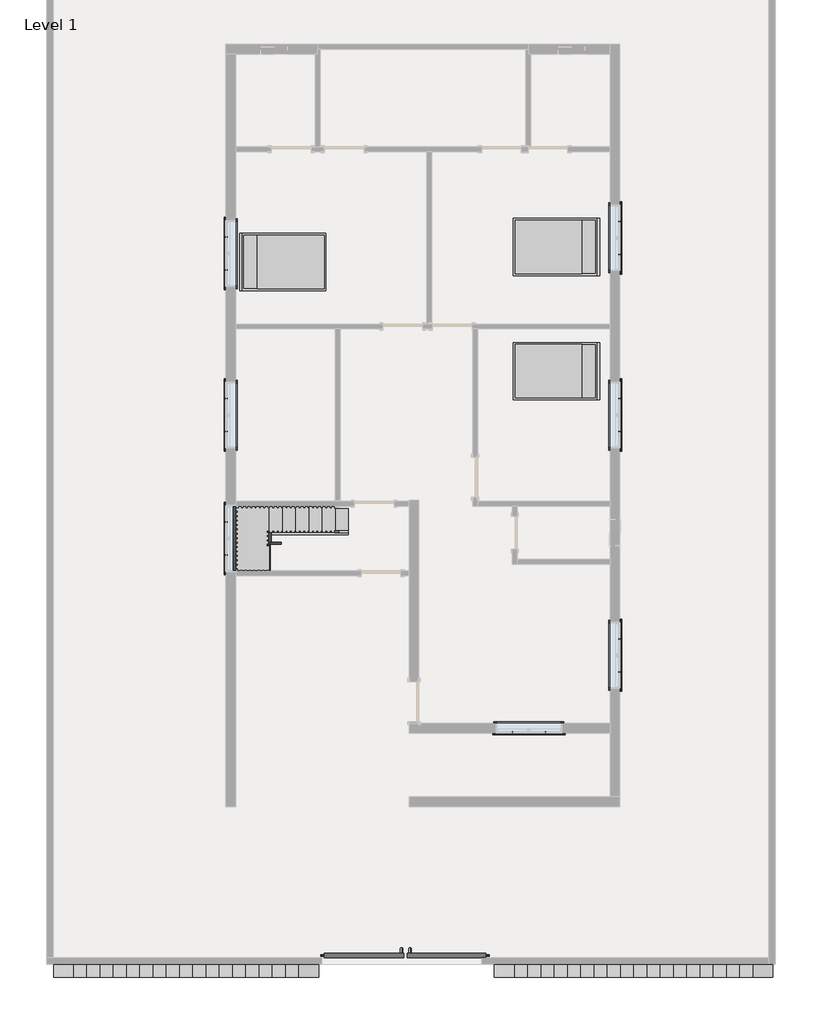
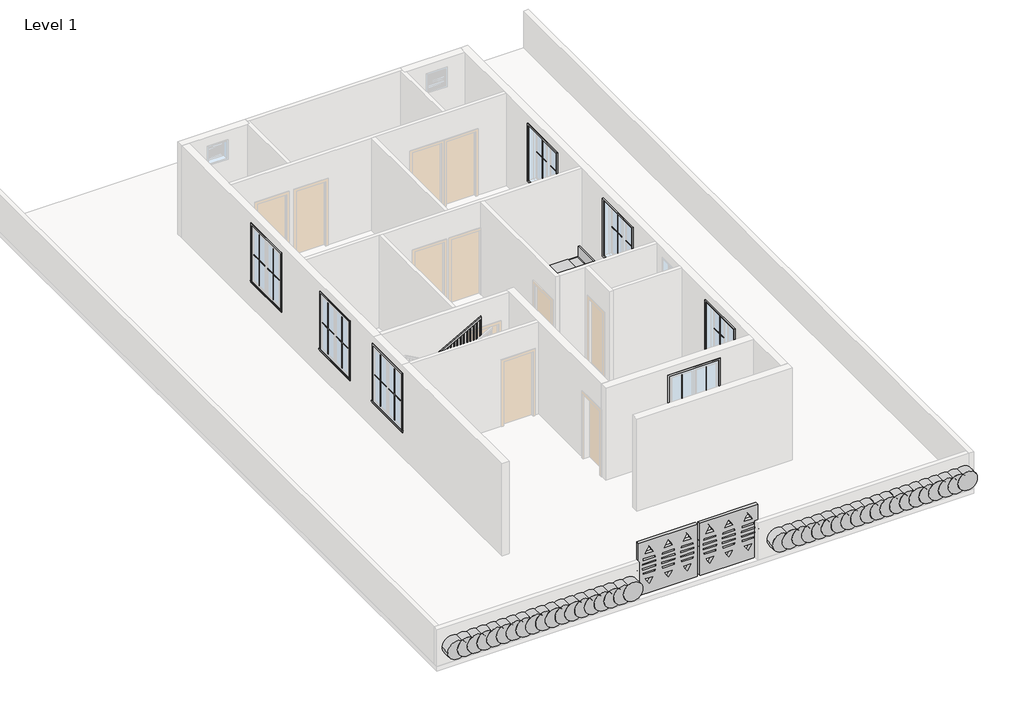
# One storey, part 3 of 3: 30 proxies, 6 members, 3 furniture elements, 1 railing, 1 stair flight.
"""IFC4 building model written with IfcOpenShell, lengths in millimetres."""

from ifc_helpers import new_model, si_unit, frame, origin, place, context, project, spatial, polyline, outline, extrude, faceted_brep, transform, mapped, element, save
from components import generic_models_477b0933, generic_models_1_generic_models_1_03ad02fd, muntin_pattern_2x2_muntin_pattern_2x2_f6a80940, muntin_pattern_2x2_muntin_pattern_2x2_09b00a1c, trim_window_exterior_flat_with_sill_698ed857, trim_window_interior_flat_picture_frame_92551a5e, bed_17739_bed_17739_15c61121, stair_flight_79800fe3

model = new_model("IFC4")

# Units and contexts
model_context = context("Model", 3, world=origin())
ifc_project = project(units=[si_unit("LENGTHUNIT", "METRE", prefix="MILLI")], contexts=[model_context])

# Site, building, storey
site = spatial("IfcSite", under=ifc_project)
building = spatial("IfcBuilding", under=site)
storey = spatial("IfcBuildingStorey", under=building, Name="Level 1", Elevation=0.0)

# Proxies
placement = place(None, origin())
generic_models_shape = generic_models_477b0933(model_context)
element("IfcBuildingElementProxy", 1, Name="Generic Models", at=placement, inside=storey, context=model_context, shape_type="MappedRepresentation", body=[
    mapped(generic_models_shape, transform((-1343.2120155, -12551.9052022, 0.0), x_axis=(-1.0, 0.0, 0.0), y_axis=(0.0, -1.0, 0.0), z_axis=(0.0, 0.0, 1.0))),
])
generic_models_1_generic_models_1_shape = generic_models_1_generic_models_1_03ad02fd(model_context)
element("IfcBuildingElementProxy", 2, Name="Generic Models 1 : Generic Models 1", ObjectType="Generic Models 1 : Generic Models 1", at=placement, inside=storey, context=model_context, shape_type="MappedRepresentation", body=[
    mapped(generic_models_1_generic_models_1_shape, transform((0.0, 0.0, 0.0), x_axis=(1.0, 0.0, 0.0), y_axis=(0.0, 1.0, 0.0), z_axis=(0.0, 0.0, 1.0))),
])
muntin_pattern_2x2_muntin_pattern_2x2_shape = muntin_pattern_2x2_muntin_pattern_2x2_f6a80940(model_context)
element("IfcBuildingElementProxy", 3, Name="Muntin Pattern_2x2 : Muntin Pattern_2x2", ObjectType="Muntin Pattern_2x2 : Muntin Pattern_2x2", at=placement, inside=storey, context=model_context, shape_type="MappedRepresentation", body=[
    mapped(muntin_pattern_2x2_muntin_pattern_2x2_shape, transform((-5778.6870155, 3260.8309309, 984.25), x_axis=(0.0, 1.0, 0.0), y_axis=(-1.0, 0.0, 0.0), z_axis=(0.0, 0.0, 1.0))),
])
element("IfcBuildingElementProxy", 4, Name="Muntin Pattern_2x2 : Muntin Pattern_2x2", ObjectType="Muntin Pattern_2x2 : Muntin Pattern_2x2", at=placement, inside=storey, context=model_context, shape_type="MappedRepresentation", body=[
    mapped(muntin_pattern_2x2_muntin_pattern_2x2_shape, transform((3270.0629845, 4381.6059309, 984.25), x_axis=(0.0, -1.0, 0.0), y_axis=(1.0, 0.0, 0.0), z_axis=(0.0, 0.0, 1.0))),
])
element("IfcBuildingElementProxy", 5, Name="Muntin Pattern_2x2 : Muntin Pattern_2x2", ObjectType="Muntin Pattern_2x2 : Muntin Pattern_2x2", at=placement, inside=storey, context=model_context, shape_type="MappedRepresentation", body=[
    mapped(muntin_pattern_2x2_muntin_pattern_2x2_shape, transform((3270.0629845, 304.9059309, 984.25), x_axis=(0.0, -1.0, 0.0), y_axis=(1.0, 0.0, 0.0), z_axis=(0.0, 0.0, 1.0))),
])
element("IfcBuildingElementProxy", 6, Name="Muntin Pattern_2x2 : Muntin Pattern_2x2", ObjectType="Muntin Pattern_2x2 : Muntin Pattern_2x2", at=placement, inside=storey, context=model_context, shape_type="MappedRepresentation", body=[
    mapped(muntin_pattern_2x2_muntin_pattern_2x2_shape, transform((3270.0629845, -5219.5940691, 984.25), x_axis=(0.0, -1.0, 0.0), y_axis=(1.0, 0.0, 0.0), z_axis=(0.0, 0.0, 1.0))),
])
element("IfcBuildingElementProxy", 7, Name="Muntin Pattern_2x2 : Muntin Pattern_2x2", ObjectType="Muntin Pattern_2x2 : Muntin Pattern_2x2", at=placement, inside=storey, context=model_context, shape_type="MappedRepresentation", body=[
    mapped(muntin_pattern_2x2_muntin_pattern_2x2_shape, transform((1563.5004845, -7380.1815691, 984.25), x_axis=(-1.0, 0.0, 0.0), y_axis=(0.0, -1.0, 0.0), z_axis=(0.0, 0.0, 1.0))),
])
element("IfcBuildingElementProxy", 8, Name="Muntin Pattern_2x2 : Muntin Pattern_2x2", ObjectType="Muntin Pattern_2x2 : Muntin Pattern_2x2", at=placement, inside=storey, context=model_context, shape_type="MappedRepresentation", body=[
    mapped(muntin_pattern_2x2_muntin_pattern_2x2_shape, transform((-5778.6870155, -3292.3690691, 984.25), x_axis=(0.0, 1.0, 0.0), y_axis=(-1.0, 0.0, 0.0), z_axis=(0.0, 0.0, 1.0))),
])
element("IfcBuildingElementProxy", 9, Name="Muntin Pattern_2x2 : Muntin Pattern_2x2", ObjectType="Muntin Pattern_2x2 : Muntin Pattern_2x2", at=placement, inside=storey, context=model_context, shape_type="MappedRepresentation", body=[
    mapped(muntin_pattern_2x2_muntin_pattern_2x2_shape, transform((-5778.6870155, -453.9190691, 984.25), x_axis=(0.0, 1.0, 0.0), y_axis=(-1.0, 0.0, 0.0), z_axis=(0.0, 0.0, 1.0))),
])
muntin_pattern_2x2_muntin_pattern_2x2_2_shape = muntin_pattern_2x2_muntin_pattern_2x2_09b00a1c(model_context)
element("IfcBuildingElementProxy", 10, Name="Muntin Pattern_2x2 : Muntin Pattern_2x2", ObjectType="Muntin Pattern_2x2 : Muntin Pattern_2x2", at=placement, inside=storey, context=model_context, shape_type="MappedRepresentation", body=[
    mapped(muntin_pattern_2x2_muntin_pattern_2x2_2_shape, transform((-5778.6870155, 4019.6559309, 984.25), x_axis=(0.0, -1.0, 0.0), y_axis=(1.0, 0.0, 0.0), z_axis=(0.0, 0.0, 1.0))),
])
element("IfcBuildingElementProxy", 11, Name="Muntin Pattern_2x2 : Muntin Pattern_2x2", ObjectType="Muntin Pattern_2x2 : Muntin Pattern_2x2", at=placement, inside=storey, context=model_context, shape_type="MappedRepresentation", body=[
    mapped(muntin_pattern_2x2_muntin_pattern_2x2_2_shape, transform((3270.0629845, 3622.7809309, 984.25), x_axis=(0.0, 1.0, 0.0), y_axis=(-1.0, 0.0, 0.0), z_axis=(0.0, 0.0, 1.0))),
])
element("IfcBuildingElementProxy", 12, Name="Muntin Pattern_2x2 : Muntin Pattern_2x2", ObjectType="Muntin Pattern_2x2 : Muntin Pattern_2x2", at=placement, inside=storey, context=model_context, shape_type="MappedRepresentation", body=[
    mapped(muntin_pattern_2x2_muntin_pattern_2x2_2_shape, transform((3270.0629845, -453.9190691, 984.25), x_axis=(0.0, 1.0, 0.0), y_axis=(-1.0, 0.0, 0.0), z_axis=(0.0, 0.0, 1.0))),
])
element("IfcBuildingElementProxy", 13, Name="Muntin Pattern_2x2 : Muntin Pattern_2x2", ObjectType="Muntin Pattern_2x2 : Muntin Pattern_2x2", at=placement, inside=storey, context=model_context, shape_type="MappedRepresentation", body=[
    mapped(muntin_pattern_2x2_muntin_pattern_2x2_2_shape, transform((3270.0629845, -5978.4190691, 984.25), x_axis=(0.0, 1.0, 0.0), y_axis=(-1.0, 0.0, 0.0), z_axis=(0.0, 0.0, 1.0))),
])
element("IfcBuildingElementProxy", 14, Name="Muntin Pattern_2x2 : Muntin Pattern_2x2", ObjectType="Muntin Pattern_2x2 : Muntin Pattern_2x2", at=placement, inside=storey, context=model_context, shape_type="MappedRepresentation", body=[
    mapped(muntin_pattern_2x2_muntin_pattern_2x2_2_shape, transform((804.6754845, -7380.1815691, 984.25), x_axis=(1.0, 0.0, 0.0), y_axis=(0.0, 1.0, 0.0), z_axis=(0.0, 0.0, 1.0))),
])
element("IfcBuildingElementProxy", 15, Name="Muntin Pattern_2x2 : Muntin Pattern_2x2", ObjectType="Muntin Pattern_2x2 : Muntin Pattern_2x2", at=placement, inside=storey, context=model_context, shape_type="MappedRepresentation", body=[
    mapped(muntin_pattern_2x2_muntin_pattern_2x2_2_shape, transform((-5778.6870155, -2533.5440691, 984.25), x_axis=(0.0, -1.0, 0.0), y_axis=(1.0, 0.0, 0.0), z_axis=(0.0, 0.0, 1.0))),
])
element("IfcBuildingElementProxy", 16, Name="Muntin Pattern_2x2 : Muntin Pattern_2x2", ObjectType="Muntin Pattern_2x2 : Muntin Pattern_2x2", at=placement, inside=storey, context=model_context, shape_type="MappedRepresentation", body=[
    mapped(muntin_pattern_2x2_muntin_pattern_2x2_2_shape, transform((-5778.6870155, 304.9059309, 984.25), x_axis=(0.0, -1.0, 0.0), y_axis=(1.0, 0.0, 0.0), z_axis=(0.0, 0.0, 1.0))),
])
trim_window_exterior_flat_with_sill_shape = trim_window_exterior_flat_with_sill_698ed857(model_context)
element("IfcBuildingElementProxy", 17, Name="Trim-Window-Exterior-Flat : with Sill", ObjectType="Trim-Window-Exterior-Flat : with Sill", at=placement, inside=storey, context=model_context, shape_type="MappedRepresentation", body=[
    mapped(trim_window_exterior_flat_with_sill_shape, transform((-5788.2120155, 3640.2434309, 2743.2), x_axis=(0.0, -1.0, 0.0), y_axis=(0.0, 0.0, 1.0), z_axis=(-1.0, 0.0, 0.0))),
])
element("IfcBuildingElementProxy", 18, Name="Trim-Window-Exterior-Flat : with Sill", ObjectType="Trim-Window-Exterior-Flat : with Sill", at=placement, inside=storey, context=model_context, shape_type="MappedRepresentation", body=[
    mapped(trim_window_exterior_flat_with_sill_shape, transform((3279.5879845, 4002.1934309, 2743.2), x_axis=(0.0, 1.0, 0.0), y_axis=(0.0, 0.0, 1.0), z_axis=(1.0, 0.0, 0.0))),
])
element("IfcBuildingElementProxy", 19, Name="Trim-Window-Exterior-Flat : with Sill", ObjectType="Trim-Window-Exterior-Flat : with Sill", at=placement, inside=storey, context=model_context, shape_type="MappedRepresentation", body=[
    mapped(trim_window_exterior_flat_with_sill_shape, transform((3279.5879845, -74.5065691, 2743.2), x_axis=(0.0, 1.0, 0.0), y_axis=(0.0, 0.0, 1.0), z_axis=(1.0, 0.0, 0.0))),
])
element("IfcBuildingElementProxy", 20, Name="Trim-Window-Exterior-Flat : with Sill", ObjectType="Trim-Window-Exterior-Flat : with Sill", at=placement, inside=storey, context=model_context, shape_type="MappedRepresentation", body=[
    mapped(trim_window_exterior_flat_with_sill_shape, transform((3279.5879845, -5599.0065691, 2743.2), x_axis=(0.0, 1.0, 0.0), y_axis=(0.0, 0.0, 1.0), z_axis=(1.0, 0.0, 0.0))),
])
element("IfcBuildingElementProxy", 21, Name="Trim-Window-Exterior-Flat : with Sill", ObjectType="Trim-Window-Exterior-Flat : with Sill", at=placement, inside=storey, context=model_context, shape_type="MappedRepresentation", body=[
    mapped(trim_window_exterior_flat_with_sill_shape, transform((1184.0879845, -7389.7065691, 2743.2), x_axis=(1.0, 0.0, 0.0), y_axis=(0.0, 0.0, 1.0), z_axis=(0.0, -1.0, 0.0))),
])
element("IfcBuildingElementProxy", 22, Name="Trim-Window-Exterior-Flat : with Sill", ObjectType="Trim-Window-Exterior-Flat : with Sill", at=placement, inside=storey, context=model_context, shape_type="MappedRepresentation", body=[
    mapped(trim_window_exterior_flat_with_sill_shape, transform((-5788.2120155, -2912.9565691, 2743.2), x_axis=(0.0, -1.0, 0.0), y_axis=(0.0, 0.0, 1.0), z_axis=(-1.0, 0.0, 0.0))),
])
element("IfcBuildingElementProxy", 23, Name="Trim-Window-Exterior-Flat : with Sill", ObjectType="Trim-Window-Exterior-Flat : with Sill", at=placement, inside=storey, context=model_context, shape_type="MappedRepresentation", body=[
    mapped(trim_window_exterior_flat_with_sill_shape, transform((-5788.2120155, -74.5065691, 2743.2), x_axis=(0.0, -1.0, 0.0), y_axis=(0.0, 0.0, 1.0), z_axis=(-1.0, 0.0, 0.0))),
])
trim_window_interior_flat_picture_frame_shape = trim_window_interior_flat_picture_frame_92551a5e(model_context)
element("IfcBuildingElementProxy", 24, Name="Trim-Window-Interior-Flat : Picture Frame", ObjectType="Trim-Window-Interior-Flat : Picture Frame", at=placement, inside=storey, context=model_context, shape_type="MappedRepresentation", body=[
    mapped(trim_window_interior_flat_picture_frame_shape, transform((-5559.6120155, 3640.2434309, 2743.2), x_axis=(0.0, 1.0, 0.0), y_axis=(0.0, 0.0, 1.0), z_axis=(1.0, 0.0, 0.0))),
])
element("IfcBuildingElementProxy", 25, Name="Trim-Window-Interior-Flat : Picture Frame", ObjectType="Trim-Window-Interior-Flat : Picture Frame", at=placement, inside=storey, context=model_context, shape_type="MappedRepresentation", body=[
    mapped(trim_window_interior_flat_picture_frame_shape, transform((3050.9879845, 4002.1934309, 2743.2), x_axis=(0.0, -1.0, 0.0), y_axis=(0.0, 0.0, 1.0), z_axis=(-1.0, 0.0, 0.0))),
])
element("IfcBuildingElementProxy", 26, Name="Trim-Window-Interior-Flat : Picture Frame", ObjectType="Trim-Window-Interior-Flat : Picture Frame", at=placement, inside=storey, context=model_context, shape_type="MappedRepresentation", body=[
    mapped(trim_window_interior_flat_picture_frame_shape, transform((3050.9879845, -74.5065691, 2743.2), x_axis=(0.0, -1.0, 0.0), y_axis=(0.0, 0.0, 1.0), z_axis=(-1.0, 0.0, 0.0))),
])
element("IfcBuildingElementProxy", 27, Name="Trim-Window-Interior-Flat : Picture Frame", ObjectType="Trim-Window-Interior-Flat : Picture Frame", at=placement, inside=storey, context=model_context, shape_type="MappedRepresentation", body=[
    mapped(trim_window_interior_flat_picture_frame_shape, transform((3050.9879845, -5599.0065691, 2743.2), x_axis=(0.0, -1.0, 0.0), y_axis=(0.0, 0.0, 1.0), z_axis=(-1.0, 0.0, 0.0))),
])
element("IfcBuildingElementProxy", 28, Name="Trim-Window-Interior-Flat : Picture Frame", ObjectType="Trim-Window-Interior-Flat : Picture Frame", at=placement, inside=storey, context=model_context, shape_type="MappedRepresentation", body=[
    mapped(trim_window_interior_flat_picture_frame_shape, transform((1184.0879845, -7161.1065691, 2743.2), x_axis=(-1.0, 0.0, 0.0), y_axis=(0.0, 0.0, 1.0), z_axis=(0.0, 1.0, 0.0))),
])
element("IfcBuildingElementProxy", 29, Name="Trim-Window-Interior-Flat : Picture Frame", ObjectType="Trim-Window-Interior-Flat : Picture Frame", at=placement, inside=storey, context=model_context, shape_type="MappedRepresentation", body=[
    mapped(trim_window_interior_flat_picture_frame_shape, transform((-5559.6120155, -2912.9565691, 2743.2), x_axis=(0.0, 1.0, 0.0), y_axis=(0.0, 0.0, 1.0), z_axis=(1.0, 0.0, 0.0))),
])
element("IfcBuildingElementProxy", 30, Name="Trim-Window-Interior-Flat : Picture Frame", ObjectType="Trim-Window-Interior-Flat : Picture Frame", at=placement, inside=storey, context=model_context, shape_type="MappedRepresentation", body=[
    mapped(trim_window_interior_flat_picture_frame_shape, transform((-5559.6120155, -74.5065691, 2743.2), x_axis=(0.0, 1.0, 0.0), y_axis=(0.0, 0.0, 1.0), z_axis=(1.0, 0.0, 0.0))),
])

# Furniture
bed_17739_bed_17739_shape = bed_17739_bed_17739_15c61121(model_context)
element("IfcFurniture", 31, ObjectType="Bed_17739 : Bed_17739", at=placement, inside=storey, context=model_context, shape_type="MappedRepresentation", body=[
    mapped(bed_17739_bed_17739_shape, transform((-4454.7120155, 3449.7434309, 0.0), x_axis=(0.0, 1.0, 0.0), y_axis=(-1.0, 0.0, 0.0), z_axis=(0.0, 0.0, 1.0))),
])
element("IfcFurniture", 32, ObjectType="Bed_17739 : Bed_17739", at=placement, inside=storey, context=model_context, shape_type="MappedRepresentation", body=[
    mapped(bed_17739_bed_17739_shape, transform((1793.6879845, 3792.6434309, 0.0), x_axis=(0.0, -1.0, 0.0), y_axis=(1.0, 0.0, 0.0), z_axis=(0.0, 0.0, 1.0))),
])
element("IfcFurniture", 33, ObjectType="Bed_17739 : Bed_17739", at=placement, inside=storey, context=model_context, shape_type="MappedRepresentation", body=[
    mapped(bed_17739_bed_17739_shape, transform((1793.6879845, 935.1434309, 0.0), x_axis=(0.0, -1.0, 0.0), y_axis=(1.0, 0.0, 0.0), z_axis=(0.0, 0.0, 1.0))),
])

# Members
element("IfcMember", 34, ObjectType="Stringer - 2\" Width", at=placement, inside=storey, context=model_context, shape_type="SweptSolid", body=[
    extrude(outline(polyline([(0.0, -2968.8120155), (207.5983948, -2968.8120155), (1195.3761726, -4746.8120155), (846.6974984, -4746.8120155), (0.0, -3222.7565183), (0.0, -2968.8120155)])), frame((0.0, -2830.4065691, 0.0), z_axis=(0.0, 1.0, 0.0), x_axis=(0.0, 0.0, 1.0)), (0.0, 0.0, 1.0), 50.8),
])
element("IfcMember", 35, ObjectType="Stringer - 2\" Width", at=placement, inside=storey, context=model_context, shape_type="SweptSolid", body=[
    extrude(outline(polyline([(-4797.6120155, -2779.6065691), (-4746.8120155, -2779.6065691), (-4746.8120155, -2995.5065691), (-4797.6120155, -2995.5065691), (-4797.6120155, -2779.6065691)])), frame((0.0, 0.0, 956.7333333), z_axis=(0.0, 0.0, 1.0), x_axis=(1.0, 0.0, 0.0)), (0.0, 0.0, 1.0), 304.8),
])
element("IfcMember", 36, ObjectType="Stringer - 2\" Width", at=placement, inside=storey, context=model_context, shape_type="SweptSolid", body=[
    extrude(outline(polyline([(1392.9317281, -4797.6120155), (1044.253054, -4797.6120155), (2060.253054, -2968.8120155), (2408.9317281, -2968.8120155), (1392.9317281, -4797.6120155)])), frame((0.0, -3046.3065691, 0.0), z_axis=(0.0, 1.0, 0.0), x_axis=(0.0, 0.0, 1.0)), (0.0, 0.0, 1.0), 50.8),
])
element("IfcMember", 37, ObjectType="Stringer - 2\" Width", at=placement, inside=storey, context=model_context, shape_type="SweptSolid", body=[
    extrude(outline(polyline([(0.0, -2968.8120155), (207.5983948, -2968.8120155), (1261.5333333, -4865.8949049), (1261.5333333, -5493.5165183), (0.0, -3222.7565183), (0.0, -2968.8120155)])), frame((0.0, -2170.0065691, 0.0), z_axis=(0.0, 1.0, 0.0), x_axis=(0.0, 0.0, 1.0)), (0.0, 0.0, 1.0), 50.8),
])
element("IfcMember", 38, ObjectType="Stringer - 2\" Width", at=placement, inside=storey, context=model_context, shape_type="SweptSolid", body=[
    extrude(outline(polyline([(-5610.4120155, -2119.2065691), (-5559.6120155, -2119.2065691), (-5559.6120155, -3674.9565691), (-5610.4120155, -3674.9565691), (-5610.4120155, -2119.2065691)])), frame((0.0, 0.0, 956.7333333), z_axis=(0.0, 0.0, 1.0), x_axis=(1.0, 0.0, 0.0)), (0.0, 0.0, 1.0), 304.8),
])
element("IfcMember", 39, ObjectType="Stringer - 2\" Width", at=placement, inside=storey, context=model_context, shape_type="SweptSolid", body=[
    extrude(outline(polyline([(956.7333333, -4955.1475127), (2060.253054, -2968.8120155), (2408.9317281, -2968.8120155), (956.7333333, -5582.7691261), (956.7333333, -4955.1475127)])), frame((0.0, -3725.7565691, 0.0), z_axis=(0.0, 1.0, 0.0), x_axis=(0.0, 0.0, 1.0)), (0.0, 0.0, 1.0), 50.8),
])

# Railing
element("IfcRailing", 40, ObjectType="Handrail - Rectangular", at=placement, inside=storey, context=model_context, shape_type="SolidModel", body=[
    faceted_brep([(-2968.8120155, -2779.6065691, 1083.7333333), (-2968.8120155, -2779.6065691, 1025.620221), (-2968.8120155, -2728.8065691, 1025.620221), (-2968.8120155, -2728.8065691, 1083.7333333), (-4721.4120155, -2779.6065691, 2057.4), (-4772.2120155, -2779.6065691, 2027.5091099), (-4772.2120155, -2728.8065691, 2027.5091099), (-4721.4120155, -2728.8065691, 2057.4), (-4721.4120155, -2779.6065691, 2099.7333333), (-4772.2120155, -2779.6065691, 2048.9333333), (-4772.2120155, -2728.8065691, 2048.9333333), (-4721.4120155, -2728.8065691, 2099.7333333), (-4797.6120155, -2779.6065691, 2099.7333333), (-4797.6120155, -2779.6065691, 2048.9333333), (-4848.4120155, -2728.8065691, 2048.9333333), (-4848.4120155, -2728.8065691, 2099.7333333), (-4797.6120155, -2855.8065691, 2099.7333333), (-4797.6120155, -2855.8065691, 2048.9333333), (-4848.4120155, -2855.8065691, 2048.9333333), (-4848.4120155, -2855.8065691, 2099.7333333), (-4797.6120155, -2970.1065691, 2099.7333333), (-4797.6120155, -3020.9065691, 2048.9333333), (-4848.4120155, -3020.9065691, 2048.9333333), (-4848.4120155, -2970.1065691, 2099.7333333), (-4797.6120155, -2970.1065691, 2311.4), (-4797.6120155, -3020.9065691, 2260.6), (-4848.4120155, -3020.9065691, 2260.6), (-4848.4120155, -2970.1065691, 2311.4), (-4797.6120155, -3046.3065691, 2311.4), (-4797.6120155, -3046.3065691, 2260.6), (-4848.4120155, -3097.1065691, 2260.6), (-4848.4120155, -3097.1065691, 2311.4), (-4721.4120155, -3046.3065691, 2311.4), (-4708.2484132, -3046.3065691, 2260.6), (-4708.2484132, -3097.1065691, 2260.6), (-4721.4120155, -3097.1065691, 2311.4), (-2968.8120155, -3046.3065691, 3285.0666667), (-2968.8120155, -3097.1065691, 3285.0666667), (-2968.8120155, -3097.1065691, 3226.9535543), (-2968.8120155, -3046.3065691, 3226.9535543)], [[[0, 1, 2, 3]], [[1, 0, 4, 5]], [[2, 1, 5, 6]], [[3, 2, 6, 7]], [[0, 3, 7, 4]], [[5, 4, 8, 9]], [[6, 5, 9, 10]], [[7, 6, 10, 11]], [[4, 7, 11, 8]], [[9, 8, 12, 13]], [[10, 9, 13, 14]], [[11, 10, 14, 15]], [[8, 11, 15, 12]], [[13, 12, 16, 17]], [[14, 13, 17, 18]], [[15, 14, 18, 19]], [[12, 15, 19, 16]], [[17, 16, 20, 21]], [[18, 17, 21, 22]], [[19, 18, 22, 23]], [[16, 19, 23, 20]], [[21, 20, 24, 25]], [[22, 21, 25, 26]], [[23, 22, 26, 27]], [[20, 23, 27, 24]], [[25, 24, 28, 29]], [[26, 25, 29, 30]], [[27, 26, 30, 31]], [[24, 27, 31, 28]], [[29, 28, 32, 33]], [[30, 29, 33, 34]], [[31, 30, 34, 35]], [[28, 31, 35, 32]], [[36, 37, 38, 39]], [[33, 32, 36, 39]], [[34, 33, 39, 38]], [[35, 34, 38, 37]], [[32, 35, 37, 36]]]),
    extrude(outline(polyline([(3207.5507765, -3003.7370155), (2201.3333333, -3003.7370155), (2201.3333333, -2984.6870155), (3218.1341099, -2984.6870155), (3207.5507765, -3003.7370155)])), frame((0.0, -3081.2315691, 0.0), z_axis=(0.0, 1.0, 0.0), x_axis=(0.0, 0.0, 1.0)), (0.0, 0.0, 1.0), 19.05),
    extrude(outline(polyline([(3151.1063321, -3105.3370155), (2201.3333333, -3105.3370155), (2201.3333333, -3086.2870155), (3161.6896654, -3086.2870155), (3151.1063321, -3105.3370155)])), frame((0.0, -3081.2315691, 0.0), z_axis=(0.0, 1.0, 0.0), x_axis=(0.0, 0.0, 1.0)), (0.0, 0.0, 1.0), 19.05),
    extrude(outline(polyline([(3094.6618876, -3206.9370155), (2201.3333333, -3206.9370155), (2201.3333333, -3187.8870155), (3105.245221, -3187.8870155), (3094.6618876, -3206.9370155)])), frame((0.0, -3081.2315691, 0.0), z_axis=(0.0, 1.0, 0.0), x_axis=(0.0, 0.0, 1.0)), (0.0, 0.0, 1.0), 19.05),
    extrude(outline(polyline([(3038.2174432, -3308.5370155), (2032.0, -3308.5370155), (2032.0, -3289.4870155), (3048.8007765, -3289.4870155), (3038.2174432, -3308.5370155)])), frame((0.0, -3081.2315691, 0.0), z_axis=(0.0, 1.0, 0.0), x_axis=(0.0, 0.0, 1.0)), (0.0, 0.0, 1.0), 19.05),
    extrude(outline(polyline([(2981.7729988, -3410.1370155), (2032.0, -3410.1370155), (2032.0, -3391.0870155), (2992.3563321, -3391.0870155), (2981.7729988, -3410.1370155)])), frame((0.0, -3081.2315691, 0.0), z_axis=(0.0, 1.0, 0.0), x_axis=(0.0, 0.0, 1.0)), (0.0, 0.0, 1.0), 19.05),
    extrude(outline(polyline([(2925.3285543, -3511.7370155), (2032.0, -3511.7370155), (2032.0, -3492.6870155), (2935.9118876, -3492.6870155), (2925.3285543, -3511.7370155)])), frame((0.0, -3081.2315691, 0.0), z_axis=(0.0, 1.0, 0.0), x_axis=(0.0, 0.0, 1.0)), (0.0, 0.0, 1.0), 19.05),
    extrude(outline(polyline([(2868.8841099, -3613.3370155), (1862.6666667, -3613.3370155), (1862.6666667, -3594.2870155), (2879.4674432, -3594.2870155), (2868.8841099, -3613.3370155)])), frame((0.0, -3081.2315691, 0.0), z_axis=(0.0, 1.0, 0.0), x_axis=(0.0, 0.0, 1.0)), (0.0, 0.0, 1.0), 19.05),
    extrude(outline(polyline([(2812.4396654, -3714.9370155), (1862.6666667, -3714.9370155), (1862.6666667, -3695.8870155), (2823.0229988, -3695.8870155), (2812.4396654, -3714.9370155)])), frame((0.0, -3081.2315691, 0.0), z_axis=(0.0, 1.0, 0.0), x_axis=(0.0, 0.0, 1.0)), (0.0, 0.0, 1.0), 19.05),
    extrude(outline(polyline([(2755.995221, -3816.5370155), (1862.6666667, -3816.5370155), (1862.6666667, -3797.4870155), (2766.5785543, -3797.4870155), (2755.995221, -3816.5370155)])), frame((0.0, -3081.2315691, 0.0), z_axis=(0.0, 1.0, 0.0), x_axis=(0.0, 0.0, 1.0)), (0.0, 0.0, 1.0), 19.05),
    extrude(outline(polyline([(2699.5507765, -3918.1370155), (1693.3333333, -3918.1370155), (1693.3333333, -3899.0870155), (2710.1341099, -3899.0870155), (2699.5507765, -3918.1370155)])), frame((0.0, -3081.2315691, 0.0), z_axis=(0.0, 1.0, 0.0), x_axis=(0.0, 0.0, 1.0)), (0.0, 0.0, 1.0), 19.05),
    extrude(outline(polyline([(2643.1063321, -4019.7370155), (1693.3333333, -4019.7370155), (1693.3333333, -4000.6870155), (2653.6896654, -4000.6870155), (2643.1063321, -4019.7370155)])), frame((0.0, -3081.2315691, 0.0), z_axis=(0.0, 1.0, 0.0), x_axis=(0.0, 0.0, 1.0)), (0.0, 0.0, 1.0), 19.05),
    extrude(outline(polyline([(2586.6618876, -4121.3370155), (1693.3333333, -4121.3370155), (1693.3333333, -4102.2870155), (2597.245221, -4102.2870155), (2586.6618876, -4121.3370155)])), frame((0.0, -3081.2315691, 0.0), z_axis=(0.0, 1.0, 0.0), x_axis=(0.0, 0.0, 1.0)), (0.0, 0.0, 1.0), 19.05),
    extrude(outline(polyline([(2530.2174432, -4222.9370155), (1524.0, -4222.9370155), (1524.0, -4203.8870155), (2540.8007765, -4203.8870155), (2530.2174432, -4222.9370155)])), frame((0.0, -3081.2315691, 0.0), z_axis=(0.0, 1.0, 0.0), x_axis=(0.0, 0.0, 1.0)), (0.0, 0.0, 1.0), 19.05),
    extrude(outline(polyline([(2473.7729988, -4324.5370155), (1524.0, -4324.5370155), (1524.0, -4305.4870155), (2484.3563321, -4305.4870155), (2473.7729988, -4324.5370155)])), frame((0.0, -3081.2315691, 0.0), z_axis=(0.0, 1.0, 0.0), x_axis=(0.0, 0.0, 1.0)), (0.0, 0.0, 1.0), 19.05),
    extrude(outline(polyline([(2417.3285543, -4426.1370155), (1524.0, -4426.1370155), (1524.0, -4407.0870155), (2427.9118876, -4407.0870155), (2417.3285543, -4426.1370155)])), frame((0.0, -3081.2315691, 0.0), z_axis=(0.0, 1.0, 0.0), x_axis=(0.0, 0.0, 1.0)), (0.0, 0.0, 1.0), 19.05),
    extrude(outline(polyline([(2360.8841099, -4527.7370155), (1354.6666667, -4527.7370155), (1354.6666667, -4508.6870155), (2371.4674432, -4508.6870155), (2360.8841099, -4527.7370155)])), frame((0.0, -3081.2315691, 0.0), z_axis=(0.0, 1.0, 0.0), x_axis=(0.0, 0.0, 1.0)), (0.0, 0.0, 1.0), 19.05),
    extrude(outline(polyline([(2304.4396654, -4629.3370155), (1354.6666667, -4629.3370155), (1354.6666667, -4610.2870155), (2315.0229988, -4610.2870155), (2304.4396654, -4629.3370155)])), frame((0.0, -3081.2315691, 0.0), z_axis=(0.0, 1.0, 0.0), x_axis=(0.0, 0.0, 1.0)), (0.0, 0.0, 1.0), 19.05),
    extrude(outline(polyline([(2247.995221, -4730.9370155), (1354.6666667, -4730.9370155), (1354.6666667, -4711.8870155), (2258.5785543, -4711.8870155), (2247.995221, -4730.9370155)])), frame((0.0, -3081.2315691, 0.0), z_axis=(0.0, 1.0, 0.0), x_axis=(0.0, 0.0, 1.0)), (0.0, 0.0, 1.0), 19.05),
    extrude(outline(polyline([(-4813.4870155, -3049.4815691), (-4813.4870155, -3068.5315691), (-4832.5370155, -3068.5315691), (-4832.5370155, -3049.4815691), (-4813.4870155, -3049.4815691)])), frame((0.0, 0.0, 1185.3333333), z_axis=(0.0, 0.0, 1.0), x_axis=(1.0, 0.0, 0.0)), (0.0, 0.0, 1.0), 1075.2666667),
    extrude(outline(polyline([(-4813.4870155, -2947.8815691), (-4813.4870155, -2966.9315691), (-4832.5370155, -2966.9315691), (-4832.5370155, -2947.8815691), (-4813.4870155, -2947.8815691)])), frame((0.0, 0.0, 1185.3333333), z_axis=(0.0, 0.0, 1.0), x_axis=(1.0, 0.0, 0.0)), (0.0, 0.0, 1.0), 863.6),
    extrude(outline(polyline([(-4813.4870155, -2846.2815691), (-4813.4870155, -2865.3315691), (-4832.5370155, -2865.3315691), (-4832.5370155, -2846.2815691), (-4813.4870155, -2846.2815691)])), frame((0.0, 0.0, 1185.3333333), z_axis=(0.0, 0.0, 1.0), x_axis=(1.0, 0.0, 0.0)), (0.0, 0.0, 1.0), 863.6),
    extrude(outline(polyline([(-4788.0870155, -2763.7315691), (-4807.1370155, -2763.7315691), (-4807.1370155, -2744.6815691), (-4788.0870155, -2744.6815691), (-4788.0870155, -2763.7315691)])), frame((0.0, 0.0, 1185.3333333), z_axis=(0.0, 0.0, 1.0), x_axis=(1.0, 0.0, 0.0)), (0.0, 0.0, 1.0), 863.6),
    extrude(outline(polyline([(1990.4674432, -4705.5370155), (1016.0, -4705.5370155), (1016.0, -4686.4870155), (1979.8841099, -4686.4870155), (1990.4674432, -4705.5370155)])), frame((0.0, -2763.7315691, 0.0), z_axis=(0.0, 1.0, 0.0), x_axis=(0.0, 0.0, 1.0)), (0.0, 0.0, 1.0), 19.05),
    extrude(outline(polyline([(1934.0229988, -4603.9370155), (1016.0, -4603.9370155), (1016.0, -4584.8870155), (1923.4396654, -4584.8870155), (1934.0229988, -4603.9370155)])), frame((0.0, -2763.7315691, 0.0), z_axis=(0.0, 1.0, 0.0), x_axis=(0.0, 0.0, 1.0)), (0.0, 0.0, 1.0), 19.05),
    extrude(outline(polyline([(1877.5785543, -4502.3370155), (1016.0, -4502.3370155), (1016.0, -4483.2870155), (1866.995221, -4483.2870155), (1877.5785543, -4502.3370155)])), frame((0.0, -2763.7315691, 0.0), z_axis=(0.0, 1.0, 0.0), x_axis=(0.0, 0.0, 1.0)), (0.0, 0.0, 1.0), 19.05),
    extrude(outline(polyline([(1821.1341099, -4400.7370155), (846.6666667, -4400.7370155), (846.6666667, -4381.6870155), (1810.5507765, -4381.6870155), (1821.1341099, -4400.7370155)])), frame((0.0, -2763.7315691, 0.0), z_axis=(0.0, 1.0, 0.0), x_axis=(0.0, 0.0, 1.0)), (0.0, 0.0, 1.0), 19.05),
    extrude(outline(polyline([(1764.6896654, -4299.1370155), (846.6666667, -4299.1370155), (846.6666667, -4280.0870155), (1754.1063321, -4280.0870155), (1764.6896654, -4299.1370155)])), frame((0.0, -2763.7315691, 0.0), z_axis=(0.0, 1.0, 0.0), x_axis=(0.0, 0.0, 1.0)), (0.0, 0.0, 1.0), 19.05),
    extrude(outline(polyline([(1708.245221, -4197.5370155), (846.6666667, -4197.5370155), (846.6666667, -4178.4870155), (1697.6618876, -4178.4870155), (1708.245221, -4197.5370155)])), frame((0.0, -2763.7315691, 0.0), z_axis=(0.0, 1.0, 0.0), x_axis=(0.0, 0.0, 1.0)), (0.0, 0.0, 1.0), 19.05),
    extrude(outline(polyline([(1651.8007765, -4095.9370155), (677.3333333, -4095.9370155), (677.3333333, -4076.8870155), (1641.2174432, -4076.8870155), (1651.8007765, -4095.9370155)])), frame((0.0, -2763.7315691, 0.0), z_axis=(0.0, 1.0, 0.0), x_axis=(0.0, 0.0, 1.0)), (0.0, 0.0, 1.0), 19.05),
    extrude(outline(polyline([(1595.3563321, -3994.3370155), (677.3333333, -3994.3370155), (677.3333333, -3975.2870155), (1584.7729988, -3975.2870155), (1595.3563321, -3994.3370155)])), frame((0.0, -2763.7315691, 0.0), z_axis=(0.0, 1.0, 0.0), x_axis=(0.0, 0.0, 1.0)), (0.0, 0.0, 1.0), 19.05),
    extrude(outline(polyline([(1538.9118876, -3892.7370155), (677.3333333, -3892.7370155), (677.3333333, -3873.6870155), (1528.3285543, -3873.6870155), (1538.9118876, -3892.7370155)])), frame((0.0, -2763.7315691, 0.0), z_axis=(0.0, 1.0, 0.0), x_axis=(0.0, 0.0, 1.0)), (0.0, 0.0, 1.0), 19.05),
    extrude(outline(polyline([(1482.4674432, -3791.1370155), (508.0, -3791.1370155), (508.0, -3772.0870155), (1471.8841099, -3772.0870155), (1482.4674432, -3791.1370155)])), frame((0.0, -2763.7315691, 0.0), z_axis=(0.0, 1.0, 0.0), x_axis=(0.0, 0.0, 1.0)), (0.0, 0.0, 1.0), 19.05),
    extrude(outline(polyline([(1426.0229988, -3689.5370155), (508.0, -3689.5370155), (508.0, -3670.4870155), (1415.4396654, -3670.4870155), (1426.0229988, -3689.5370155)])), frame((0.0, -2763.7315691, 0.0), z_axis=(0.0, 1.0, 0.0), x_axis=(0.0, 0.0, 1.0)), (0.0, 0.0, 1.0), 19.05),
    extrude(outline(polyline([(1369.5785543, -3587.9370155), (508.0, -3587.9370155), (508.0, -3568.8870155), (1358.995221, -3568.8870155), (1369.5785543, -3587.9370155)])), frame((0.0, -2763.7315691, 0.0), z_axis=(0.0, 1.0, 0.0), x_axis=(0.0, 0.0, 1.0)), (0.0, 0.0, 1.0), 19.05),
    extrude(outline(polyline([(1313.1341099, -3486.3370155), (338.6666667, -3486.3370155), (338.6666667, -3467.2870155), (1302.5507765, -3467.2870155), (1313.1341099, -3486.3370155)])), frame((0.0, -2763.7315691, 0.0), z_axis=(0.0, 1.0, 0.0), x_axis=(0.0, 0.0, 1.0)), (0.0, 0.0, 1.0), 19.05),
    extrude(outline(polyline([(1256.6896654, -3384.7370155), (338.6666667, -3384.7370155), (338.6666667, -3365.6870155), (1246.1063321, -3365.6870155), (1256.6896654, -3384.7370155)])), frame((0.0, -2763.7315691, 0.0), z_axis=(0.0, 1.0, 0.0), x_axis=(0.0, 0.0, 1.0)), (0.0, 0.0, 1.0), 19.05),
    extrude(outline(polyline([(1200.245221, -3283.1370155), (338.6666667, -3283.1370155), (338.6666667, -3264.0870155), (1189.6618876, -3264.0870155), (1200.245221, -3283.1370155)])), frame((0.0, -2763.7315691, 0.0), z_axis=(0.0, 1.0, 0.0), x_axis=(0.0, 0.0, 1.0)), (0.0, 0.0, 1.0), 19.05),
    extrude(outline(polyline([(1143.8007765, -3181.5370155), (169.3333333, -3181.5370155), (169.3333333, -3162.4870155), (1133.2174432, -3162.4870155), (1143.8007765, -3181.5370155)])), frame((0.0, -2763.7315691, 0.0), z_axis=(0.0, 1.0, 0.0), x_axis=(0.0, 0.0, 1.0)), (0.0, 0.0, 1.0), 19.05),
    extrude(outline(polyline([(1087.3563321, -3079.9370155), (169.3333333, -3079.9370155), (169.3333333, -3060.8870155), (1076.7729988, -3060.8870155), (1087.3563321, -3079.9370155)])), frame((0.0, -2763.7315691, 0.0), z_axis=(0.0, 1.0, 0.0), x_axis=(0.0, 0.0, 1.0)), (0.0, 0.0, 1.0), 19.05),
    extrude(outline(polyline([(-4813.4870155, -3062.1815691), (-4813.4870155, -3081.2315691), (-4832.5370155, -3081.2315691), (-4832.5370155, -3062.1815691), (-4813.4870155, -3062.1815691)])), frame((0.0, 0.0, 1185.3333333), z_axis=(0.0, 0.0, 1.0), x_axis=(1.0, 0.0, 0.0)), (0.0, 0.0, 1.0), 1075.2666667),
    extrude(outline(polyline([(-4813.4870155, -2763.7315691), (-4832.5370155, -2763.7315691), (-4832.5370155, -2744.6815691), (-4813.4870155, -2744.6815691), (-4813.4870155, -2763.7315691)])), frame((0.0, 0.0, 1185.3333333), z_axis=(0.0, 0.0, 1.0), x_axis=(1.0, 0.0, 0.0)), (0.0, 0.0, 1.0), 863.6),
    extrude(outline(polyline([(3216.370221, -2987.8620155), (2201.3333333, -2987.8620155), (2201.3333333, -2968.8120155), (3226.9535543, -2968.8120155), (3216.370221, -2987.8620155)])), frame((0.0, -3081.2315691, 0.0), z_axis=(0.0, 1.0, 0.0), x_axis=(0.0, 0.0, 1.0)), (0.0, 0.0, 1.0), 19.05),
    extrude(outline(polyline([(1036.2035543, -2987.8620155), (169.3333333, -2987.8620155), (169.3333333, -2968.8120155), (1025.620221, -2968.8120155), (1036.2035543, -2987.8620155)])), frame((0.0, -2763.7315691, 0.0), z_axis=(0.0, 1.0, 0.0), x_axis=(0.0, 0.0, 1.0)), (0.0, 0.0, 1.0), 19.05),
])

# Stair flight
stair_flight_shape = stair_flight_79800fe3(model_context)
element("IfcStairFlight", 41, ObjectType="2\" Tread 1\" Nosing 1/4\" Riser", at=placement, inside=storey, context=model_context, shape_type="MappedRepresentation", body=[
    mapped(stair_flight_shape, transform((0.0, 0.0, 0.0), x_axis=(1.0, 0.0, 0.0), y_axis=(0.0, 1.0, 0.0), z_axis=(0.0, 0.0, 1.0))),
])

save(model, "model.ifc")

# Revit data of these elements
# Type
#   Default Elevation = 0
# Type "Muntin Pattern_2x2 : Muntin Pattern_2x2"
#   Width [instance default] = 4' - 0"
#   Thickness = 0' - 0 1/2"
#   Height [instance default] = 4' - 0"
#   Distance = 0' - 0 3/4"
#   Interior Material [instance default] = none
#   Exterior Material [instance default] = none
#   Default Elevation = 0
# Type "Trim-Window-Exterior-Flat : with Sill"
#   Trim Width = 0' - 2 1/4"
#   Trim Thickness_Picture Frame = 0' - 1 1/4"
#   Trim Thickness_with Sill = 0' - 0 3/4"
#   Sill Thickness = 0' - 1 1/4"
#   Opening Width [instance default] = 2' - 0"
#   Opening Height [instance default] = 3' - 0"
#   Default Elevation = 4' - 0"
#   Sill = yes
#   Picture Frame = no
#   Trim Material [instance default] = none
# Type "Trim-Window-Interior-Flat : Picture Frame"
#   Trim Thickness_Picture Frame = 0' - 1 1/4"
#   Trim Width = 0' - 2 1/4"
#   Trim Thickness_with Sill = 0' - 0 3/4"
#   Sill Thickness = 0' - 1 1/4"
#   Opening Width [instance default] = 2' - 0"
#   Opening Height [instance default] = 3' - 0"
#   Default Elevation = 4' - 0"
#   Sill = no
#   Picture Frame = yes
#   Trim Material [instance default] = none
# Type "Bed_17739 : Bed_17739"
#   Default Elevation = 0
# Type "Handrail - Rectangular"
#   Assembly Code = "C2010400"
#   built-in parameter 1008612 = 0.0416667 (stored number, unit not read)
#   built-in parameter 1008611 = 0.0416667 (stored number, unit not read)
#   built-in parameter 1008609 = 0.333333 (stored number, unit not read)
#   built-in parameter 1008604 = 0.166667 (stored number, unit not read)
#   built-in parameter 1008603 = 0.166667 (stored number, unit not read)
#   Railing Height = 3' - 0"
#   built-in parameter 1008630 = 2
#   built-in parameter 1008610 = 2
#   built-in parameter 1008618 = Baluster - Square : 3/4"
# Element 1 (IfcBuildingElementProxy)
#   Phase Created = New Construction
# Element 2 (IfcBuildingElementProxy, "Generic Models 1 : Generic Models 1")
#   Phase Created = New Construction
#   Materials on its faces: "Brick, Soldier Course"
# Elements 3, 4, 5, 6, 7, 8, 9, 10, 11, 12, 13, 14, 15, 16 (IfcBuildingElementProxy, "Muntin Pattern_2x2 : Muntin Pattern_2x2")
#   Width = 2' - 0 5/8"
#   Height = 5' - 6 1/2"
#   Interior Material = Wood - Stained
#   Exterior Material = Clad - White
#   Phase Created = New Construction
#   Materials on its faces: "Clad - White", "Wood - Stained"
# Elements 17, 18, 19, 20, 21, 22, 23 (IfcBuildingElementProxy, "Trim-Window-Exterior-Flat : with Sill")
#   Opening Width = 5' - 0"
#   Opening Height = 6' - 0"
#   Trim Material = Clad - White
#   Phase Created = New Construction
#   Materials on its faces: "Clad - White"
# Elements 24, 25, 26, 27, 28, 29, 30 (IfcBuildingElementProxy, "Trim-Window-Interior-Flat : Picture Frame")
#   Opening Width = 5' - 0"
#   Opening Height = 6' - 0"
#   Trim Material = Wood - Stained
#   Phase Created = New Construction
#   Materials on its faces: "Wood - Stained"
# Elements 31, 32, 33 (IfcFurniture, "Bed_17739 : Bed_17739")
#   Phase Created = New Construction
#   Materials on its faces: "legs", "sheets", "bed frame", "Blanket"
# Elements 34, 35, 36, 37, 38, 39 (IfcMember, "Stringer - 2\" Width")
#   Phase Created = New Construction
# Element 40 (IfcRailing, "Handrail - Rectangular")
#   Phase Created = New Construction
# Element 41 (IfcStairFlight, "2\" Tread 1\" Nosing 1/4\" Riser")
#   Phase Created = New Construction
# Materials
#   "Brick, Soldier Course": class "Masonry", colour RGB 170 98 104, transparency 0, Description = "Common brick soldier coursed", Cost = 0
#   "Clad - White": class "Wood", colour RGB 242 242 238, transparency 0, Cost = 0
#   "Wood - Stained": class "Wood", colour RGB 224 178 126, transparency 0, Cost = 0
#   "legs": colour RGB 90 73 37, transparency 0, Cost = 0
#   "sheets": colour RGB 200 195 176, transparency 0, Cost = 0
#   "bed frame": colour RGB 90 73 37, transparency 0, Cost = 0
#   "Blanket": class "System", colour RGB 59 0 1, transparency 0, Cost = 0
